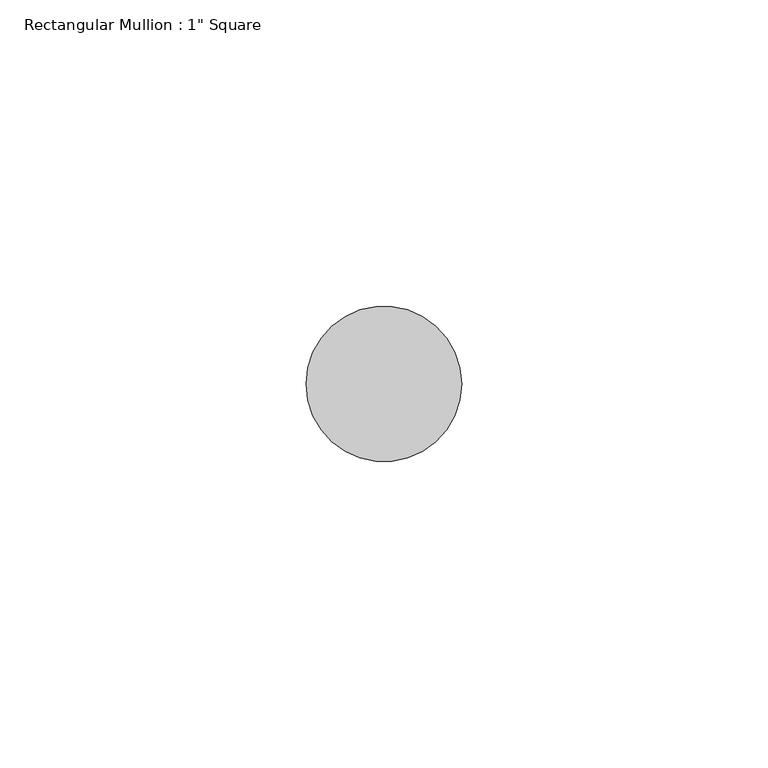
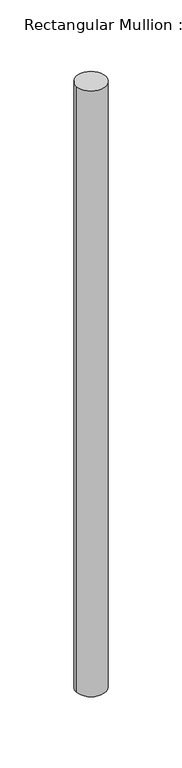
"""IFC4 building model written with IfcOpenShell, lengths in millimetres: member geometry."""

from ifc_helpers import new_model, si_unit, point, frame, origin, origin_2d, place, context, project, spatial, circle_curve, trimmed, segment, composite_curve, outline, extrude, source, transform, mapped, element, save


def member_11e54509(model_context):
    return source(origin(), model_context, "Body", "SweptSolid", [
        extrude(outline(composite_curve([segment(trimmed(circle_curve(origin_2d(), 12.7), [point((12.7, 0.0))], [point((-12.7, 0.0))], False, "CARTESIAN"), True, "CONTINUOUS"), segment(trimmed(circle_curve(origin_2d(), 12.7), [point((-12.7, 0.0))], [point((12.7, 0.0))], False, "CARTESIAN"), True, "CONTINUOUS")], self_intersect=False)), frame((0.0, 0.0, -546.1), z_axis=(0.0, 0.0, 1.0), x_axis=(1.0, 0.0, 0.0)), (0.0, 0.0, 1.0), 546.1),
    ])


if __name__ == "__main__":
    model = new_model("IFC4")
    model_context = context("Model", 3, world=origin())
    ifc_project = project(units=[si_unit("LENGTHUNIT", "METRE", prefix="MILLI")], contexts=[model_context])
    site = spatial("IfcSite", under=ifc_project)
    building = spatial("IfcBuilding", under=site)
    placement = place(None, origin())
    member_shape = member_11e54509(model_context)
    element("IfcMember", 1, ObjectType="Rectangular Mullion : 1\" Square", at=placement, inside=building, context=model_context, shape_type="MappedRepresentation", body=[
        mapped(member_shape, transform((0.0, 0.0, 0.0), x_axis=(1.0, 0.0, 0.0), y_axis=(0.0, 1.0, 0.0), z_axis=(0.0, 0.0, 1.0))),
    ])
    save(model, "model.ifc")

# Revit data of these elements
# Type "Rectangular Mullion : 1\" Square"
#   built-in parameter 1007350 = 0.0416667 (stored number, unit not read)
# Element 1 (IfcMember, "Rectangular Mullion : 1\" Square")
#   Materials on its faces: "Aluminum"
# Materials
#   "Aluminum": class "Metal", colour RGB 247 247 247, transparency 0, Description = "Aluminum 6061", Cost = 0
